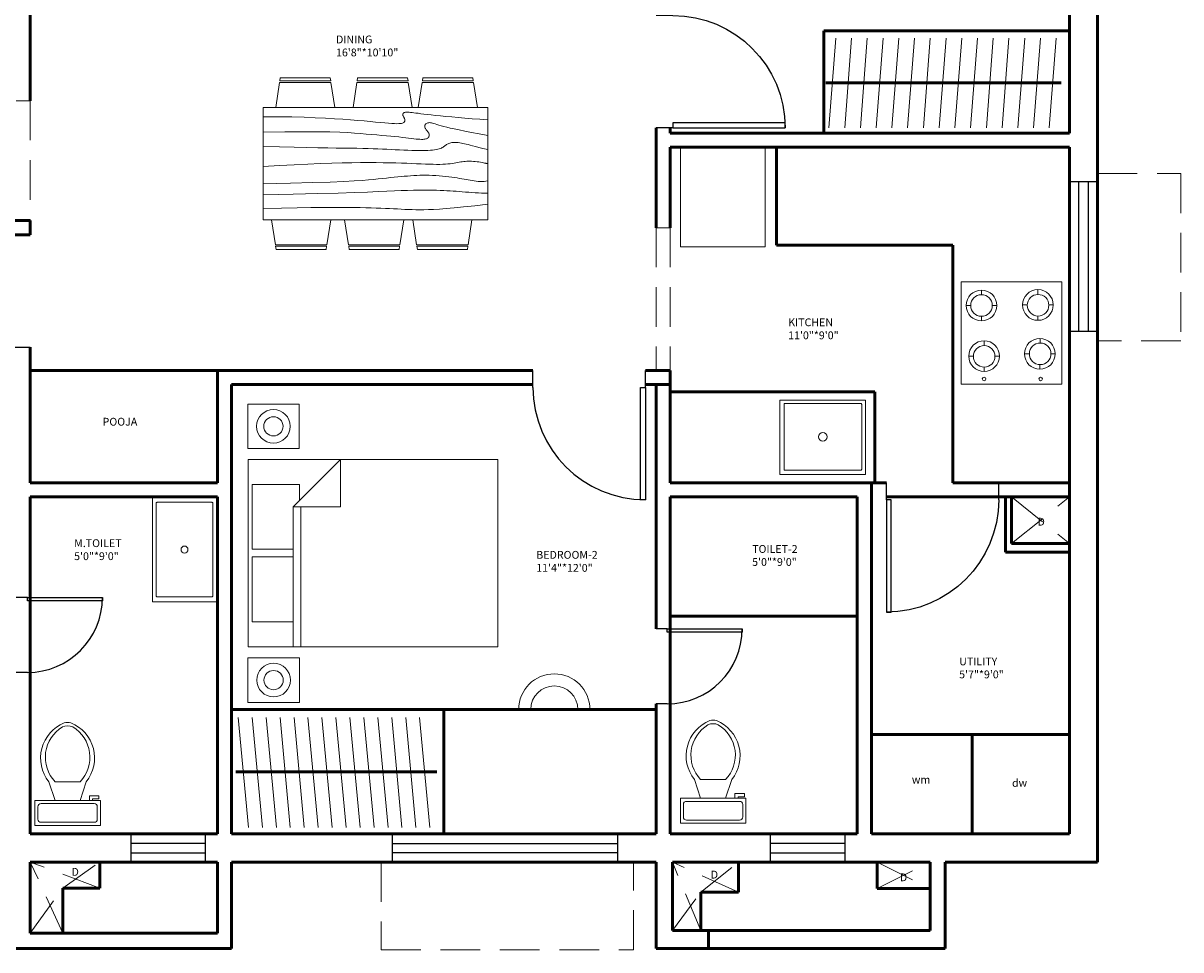
# Model space of a CAD drawing. Units: inches. Extents: x 291 to 2631, y 456 to 2623.
# Tile 21 of 22: x 2205 to 2576, y 2128 to 2425. Entities that reach past the tile are written whole.
import ezdxf

# ---------------------------------------------------------------- set-up
doc = ezdxf.new("R2010")
doc.units = ezdxf.units.IN
doc.linetypes.add('DASHED', pattern=[19.05, 12.7, -6.35])
for name, color, linetype, lineweight in [('A-ANNO-TEXT', 3, 'Continuous', 25), ('A-AREA-IDEN', 7, 'Continuous', 25), ('A-DOOR', 3, 'Continuous', 25), ('A-EQPM', 8, 'Continuous', 18), ('A-FLOR-FIXT', 9, 'Continuous', 18), ('A-FLOR-OVHD', 1, 'DASHED', 18), ('A-FURN', 8, 'Continuous', 18), ('A-GLAZ', 4, 'Continuous', 25), ('A-WALL', 7, 'Continuous', 50)]:
    doc.layers.add(name, color=color, linetype=linetype, lineweight=lineweight)
doc.styles.get("Standard").update_dxf_attribs({"font": 'arial.ttf'})

# ---------------------------------------------------------------- blocks, each defined once
blk = doc.blocks.new('*U2')
for p, q in [((0, 0), (0, -6)), ((40, 0), (40, -6))]:
    blk.add_line(p, q)
blk.add_lwpolyline([(0, 0), (0, 40), (1.75, 40), (1.75, 0)], close=True)
blk.add_arc((0, 0), 40, 0, 90)
blk = doc.blocks.new('Bed - Queen')
for p, q in [((0, -80.00003), (0, 0)), ((0, 0), (59.99999, 0)), ((59.99999, 0), (59.99999, -80.00003)), ((7.99999, -1.2), (28.79998, -1.2)), ((7.99999, -14.4), (7.99999, -1.2)), ((28.79998, -1.2), (28.79998, -14.4)), ((31.19999, -1.2), (51.99999, -1.2)), ((31.19999, -14.4), (31.19999, -1.2)), ((51.99999, -1.2), (51.99999, -16.4)), ((0, -14.4), (44.8, -14.4)), ((59.99999, -29.6), (44.8, -14.4)), ((44.8, -14.4), (44.8, -29.6)), ((44.8, -16.8), (0, -16.8)), ((51.99999, -16.4), (46.79936, -16.4)), ((44.8, -29.6), (59.99999, -29.6)), ((59.99999, -80.00003), (0, -80.00003))]:
    blk.add_line(p, q)
blk = doc.blocks.new('Toilet - top')
for p, q in [((9.5, -6), (9.5, -2)), ((-10, -8.5), (-8, -8.5)), ((-10, -9.5), (-10, -8.5)), ((-7, -9.5), (-10, -9.5)), ((-8, -8.5), (-8, -8)), ((-7, -8), (-7, -9.5)), ((-4, -8), (-6, -14)), ((4, -8), (6, -14)), ((4, -14), (-4, -14))]:
    blk.add_line(p, q)
blk.add_lwpolyline([(10.5, -8), (10.5, 0), (-10.5, 0), (-10.5, -8)], close=True)
for points in [[(-9.5, -2), (-9.5, -6)], [(8.5, -1), (-8.5, -1)], [(-8.5, -7), (8.5, -7)]]:
    blk.add_lwpolyline(points)
for centre, radius, start, end in [((-8.62, -1.88), 0.884, 81.8699, 188.1301), ((8.62, -1.88), 0.884, 351.8699, 98.1301), ((-8.62, -6.12), 0.884, 171.8699, 278.1301), ((8.62, -6.12), 0.884, 261.8699, 8.1301), ((3.52, -21.58), 12.17, 141.4691, 247.9714), ((4.2, -21.82), 11.33, 136.3677, 238.9468), ((-3.52, -21.58), 12.17, 292.0284, 38.5307), ((-4.2, -21.82), 11.33, 301.053, 43.6321), ((0, -27.88), 4, 245.7318, 294.2682), ((0, -29), 4, 254.8605, 285.1395)]:
    blk.add_arc(centre, radius, start, end)
blk = doc.blocks.new('WIN-1800')
for p, q in [((0, 9), (72, 9)), ((0, 0), (0, 9)), ((72, 9), (72, 0)), ((0, 6), (72, 6)), ((72, 3), (0, 3)), ((72, 0), (0, 0))]:
    blk.add_line(p, q)
blk = doc.blocks.new('WIN-1200')
for p, q in [((0, 0), (0, 48)), ((0, 48), (9, 48)), ((3, 0), (3, 48)), ((6, 48), (6, 0)), ((9, 48), (9, 0)), ((9, 0), (0, 0))]:
    blk.add_line(p, q)
blk = doc.blocks.new('COOKTOP')
for p, q in [((6.54, 28.68), (6.54, 30.14)), ((24.62, 30.31), (24.62, 28.76)), ((1.62, 25.22), (3.08, 25.22)), ((10, 25.22), (11.46, 25.22)), ((19.7, 25.39), (21.21, 25.39)), ((28.13, 25.39), (29.54, 25.39)), ((6.54, 21.76), (6.54, 20.3)), ((24.62, 21.83), (24.62, 20.47)), ((7.38, 13.92), (7.38, 12.38)), ((25.35, 14.65), (25.34, 13.21)), ((2.46, 9), (3.95, 9)), ((10.87, 9), (12.3, 9)), ((20.32, 9.73), (21.89, 9.73)), ((28.81, 9.73), (30.16, 9.73)), ((7.38, 5.46), (7.38, 4.08)), ((25.26, 6.28), (25.24, 4.81))]:
    blk.add_line(p, q)
blk.add_lwpolyline([(0, 32.79), (32.25, 32.79), (32.25, 0), (0, 0)], close=True)
for centre, radius in [((6.54, 25.22), 4.92), ((24.62, 25.39), 4.92), ((6.54, 25.22), 3.46), ((24.67, 25.29), 3.46), ((7.38, 9), 4.92), ((7.41, 8.92), 3.46), ((25.24, 9.73), 4.92), ((25.35, 9.74), 3.46), ((7.38, 1.69), 0.572), ((25.5, 1.69), 0.572)]:
    blk.add_circle(centre, radius)
blk = doc.blocks.new('WIN-600')
for p, q in [((24, 9), (0, 9)), ((0, 9), (0, 0)), ((24, 0), (24, 9)), ((24, 6), (0, 6)), ((0, 3), (24, 3)), ((0, 0), (24, 0))]:
    blk.add_line(p, q)

msp = doc.modelspace()

# ---------------------------------------------------------------- linework, layer by layer
at = {"layer": 'A-FLOR-OVHD'}
for p, q in [((2202.49, 2400.18), (2206.99, 2400.18)), ((2206.99, 2400.18), (2206.99, 2361.74)), ((2548.99, 2376.89), (2575.66, 2376.89)), ((2575.66, 2376.89), (2575.66, 2323.27)), ((2407.49, 2359.49), (2411.99, 2359.49)), ((2407.49, 2359.49), (2407.49, 2313.74)), ((2411.99, 2359.49), (2411.99, 2313.74)), ((2575.66, 2323.27), (2548.99, 2323.27)), ((2521.43, 2273.24), (2539.99, 2258.27)), ((2521.43, 2258.27), (2539.99, 2273.24)), ((2217.38, 2133.51), (2206.99, 2156.24)), ((2229.27, 2147.9), (2206.99, 2156.24)), ((2217.38, 2147.9), (2229.27, 2156.24)), ((2319.38, 2156.24), (2319.38, 2128.12)), ((2400.25, 2128.12), (2400.25, 2156.24)), ((2421.83, 2134.3), (2412.72, 2156.24)), ((2433.87, 2146.62), (2412.72, 2156.24)), ((2421.83, 2146.62), (2433.87, 2156.24)), ((2478.37, 2156.24), (2495.34, 2147.73)), ((2478.37, 2147.73), (2495.34, 2156.24)), ((2206.99, 2133.51), (2217.38, 2147.9)), ((2412.72, 2134.3), (2421.83, 2146.62)), ((2319.38, 2128.12), (2400.25, 2128.12))]:
    msp.add_line(p, q, dxfattribs=at)
at = {"layer": 'A-FURN'}
for p, q in [((2462.9, 2391.52), (2465.11, 2420.17)), ((2467.95, 2391.52), (2470.15, 2420.17)), ((2472.99, 2391.52), (2475.2, 2420.17)), ((2478.03, 2391.52), (2480.24, 2420.17)), ((2483.08, 2391.52), (2485.28, 2420.17)), ((2488.12, 2391.52), (2490.33, 2420.17)), ((2493.16, 2391.52), (2495.37, 2420.17)), ((2498.21, 2391.52), (2500.41, 2420.17)), ((2503.25, 2391.52), (2505.46, 2420.17)), ((2508.29, 2391.52), (2510.5, 2420.17)), ((2513.34, 2391.52), (2515.54, 2420.17)), ((2518.38, 2391.52), (2520.59, 2420.17)), ((2523.42, 2391.52), (2525.63, 2420.17)), ((2528.47, 2391.52), (2530.67, 2420.17)), ((2533.51, 2391.52), (2535.72, 2420.17)), ((2287.1, 2407.55), (2286.95, 2406.55)), ((2287.1, 2407.55), (2303.1, 2407.55)), ((2303.26, 2406.55), (2303.1, 2407.55)), ((2311.88, 2407.55), (2311.73, 2406.55)), ((2311.88, 2407.55), (2327.88, 2407.55)), ((2328.04, 2406.55), (2327.88, 2407.55)), ((2332.79, 2407.55), (2332.63, 2406.55)), ((2332.79, 2407.55), (2348.79, 2407.55)), ((2348.94, 2406.55), (2348.79, 2407.55)), ((2286.87, 2406.05), (2285.62, 2398.05)), ((2286.87, 2406.05), (2303.34, 2406.05)), ((2303.26, 2406.55), (2286.95, 2406.55)), ((2304.59, 2398.05), (2303.34, 2406.05)), ((2311.65, 2406.05), (2310.4, 2398.05)), ((2311.65, 2406.05), (2328.12, 2406.05)), ((2328.04, 2406.55), (2311.73, 2406.55)), ((2329.37, 2398.05), (2328.12, 2406.05)), ((2332.55, 2406.05), (2331.3, 2398.05)), ((2332.56, 2406.05), (2349.03, 2406.05)), ((2348.94, 2406.55), (2332.63, 2406.55)), ((2350.27, 2398.05), (2349.02, 2406.05)), ((2353.58, 2398.05), (2281.58, 2398.05)), ((2281.58, 2398.05), (2281.58, 2362.05)), ((2353.58, 2362.05), (2353.58, 2398.05)), ((2281.58, 2362.05), (2353.58, 2362.05)), ((2285.53, 2354.05), (2284.28, 2362.05)), ((2303.25, 2362.05), (2302, 2354.05)), ((2308.94, 2354.05), (2307.69, 2362.05)), ((2326.66, 2362.05), (2325.41, 2354.05)), ((2330.79, 2354.05), (2329.54, 2362.05)), ((2348.51, 2362.05), (2347.26, 2354.05)), ((2285.54, 2354.05), (2302, 2354.05)), ((2285.77, 2352.55), (2285.61, 2353.55)), ((2301.92, 2353.55), (2285.61, 2353.55)), ((2285.77, 2352.55), (2301.77, 2352.55)), ((2301.92, 2353.55), (2301.77, 2352.55)), ((2308.95, 2354.05), (2325.42, 2354.05)), ((2309.18, 2352.55), (2309.02, 2353.55)), ((2325.34, 2353.55), (2309.03, 2353.55)), ((2309.18, 2352.55), (2325.18, 2352.55)), ((2325.34, 2353.55), (2325.18, 2352.55)), ((2330.79, 2354.05), (2347.26, 2354.05)), ((2331.03, 2352.55), (2330.87, 2353.55)), ((2347.18, 2353.55), (2330.87, 2353.55)), ((2331.03, 2352.55), (2347.03, 2352.55)), ((2347.18, 2353.55), (2347.03, 2352.55)), ((2273.61, 2202.53), (2276.89, 2167.35)), ((2278.09, 2202.53), (2281.36, 2167.35)), ((2282.56, 2202.53), (2285.83, 2167.35)), ((2287.03, 2202.53), (2290.3, 2167.35)), ((2291.5, 2202.53), (2294.78, 2167.35)), ((2295.97, 2202.53), (2299.25, 2167.35)), ((2300.44, 2202.53), (2303.72, 2167.35)), ((2304.92, 2202.53), (2308.19, 2167.35)), ((2309.39, 2202.53), (2312.66, 2167.35)), ((2313.86, 2202.53), (2317.13, 2167.35)), ((2318.33, 2202.53), (2321.61, 2167.35)), ((2322.8, 2202.53), (2326.08, 2167.35)), ((2327.28, 2202.53), (2330.55, 2167.35)), ((2331.75, 2202.53), (2335.02, 2167.35))]:
    msp.add_line(p, q, dxfattribs=at)
for points in [[(2281.58, 2395.05), (2286.4, 2395.02), (2290.77, 2394.96), (2294.73, 2394.86), (2298.3, 2394.73), (2301.54, 2394.58), (2304.48, 2394.41), (2307.16, 2394.23), (2309.62, 2394.05), (2311.89, 2393.86), (2313.98, 2393.68), (2315.88, 2393.5), (2317.62, 2393.34), (2319.17, 2393.19), (2320.56, 2393.06), (2321.78, 2392.96), (2322.83, 2392.88), (2323.72, 2392.83), (2324.46, 2392.81), (2325.07, 2392.82), (2325.56, 2392.86), (2325.95, 2392.92), (2326.25, 2393), (2326.48, 2393.1), (2326.66, 2393.21), (2326.8, 2393.34), (2326.9, 2393.49), (2326.97, 2393.64), (2327.01, 2393.81), (2327.02, 2393.97), (2327, 2394.14), (2326.97, 2394.3), (2326.91, 2394.46), (2326.84, 2394.62), (2326.76, 2394.76), (2326.68, 2394.9), (2326.59, 2395.04), (2326.51, 2395.17), (2326.43, 2395.29), (2326.37, 2395.42), (2326.33, 2395.55), (2326.31, 2395.67), (2326.31, 2395.79), (2326.34, 2395.91), (2326.39, 2396.02), (2326.47, 2396.13), (2326.56, 2396.23), (2326.68, 2396.31), (2326.83, 2396.38), (2327, 2396.43), (2327.2, 2396.47), (2327.43, 2396.5), (2327.7, 2396.5), (2328.03, 2396.5), (2328.4, 2396.47), (2328.83, 2396.43), (2329.33, 2396.38), (2329.9, 2396.31), (2330.55, 2396.22), (2331.29, 2396.13), (2332.15, 2396.01), (2333.12, 2395.89), (2334.22, 2395.76), (2335.47, 2395.61), (2336.87, 2395.46), (2338.44, 2395.3), (2340.17, 2395.14), (2342.05, 2394.96), (2344.08, 2394.79), (2346.26, 2394.6), (2348.57, 2394.42), (2351.01, 2394.23), (2353.58, 2394.05)], [(2281.58, 2390.05), (2288.6, 2390.19), (2294.41, 2390.25), (2299.16, 2390.24), (2303.01, 2390.18), (2306.14, 2390.08), (2308.7, 2389.94), (2310.86, 2389.79), (2312.79, 2389.63), (2314.61, 2389.48), (2316.35, 2389.33), (2318.02, 2389.19), (2319.61, 2389.06), (2321.11, 2388.93), (2322.52, 2388.8), (2323.85, 2388.67), (2325.08, 2388.55), (2326.22, 2388.42), (2327.27, 2388.3), (2328.23, 2388.18), (2329.11, 2388.08), (2329.91, 2387.98), (2330.62, 2387.9), (2331.26, 2387.84), (2331.83, 2387.8), (2332.33, 2387.78), (2332.76, 2387.78), (2333.13, 2387.8), (2333.45, 2387.85), (2333.73, 2387.91), (2333.96, 2388), (2334.16, 2388.1), (2334.33, 2388.21), (2334.47, 2388.34), (2334.59, 2388.49), (2334.69, 2388.65), (2334.76, 2388.82), (2334.8, 2388.99), (2334.81, 2389.17), (2334.79, 2389.36), (2334.75, 2389.55), (2334.67, 2389.73), (2334.57, 2389.92), (2334.44, 2390.11), (2334.31, 2390.3), (2334.17, 2390.48), (2334.02, 2390.67), (2333.88, 2390.86), (2333.75, 2391.05), (2333.63, 2391.23), (2333.53, 2391.42), (2333.45, 2391.6), (2333.4, 2391.79), (2333.38, 2391.96), (2333.38, 2392.14), (2333.42, 2392.3), (2333.5, 2392.46), (2333.61, 2392.61), (2333.76, 2392.75), (2333.94, 2392.88), (2334.15, 2392.98), (2334.39, 2393.06), (2334.66, 2393.12), (2334.94, 2393.14), (2335.25, 2393.13), (2335.57, 2393.08), (2335.92, 2392.99), (2336.32, 2392.88), (2336.77, 2392.73), (2337.3, 2392.56), (2337.91, 2392.36), (2338.63, 2392.15), (2339.45, 2391.92), (2340.42, 2391.68), (2341.54, 2391.42), (2342.86, 2391.13), (2344.41, 2390.81), (2346.22, 2390.45), (2348.33, 2390.04), (2350.77, 2389.57), (2353.58, 2389.05)], [(2281.58, 2385.55), (2286.86, 2385.38), (2291.51, 2385.26), (2295.58, 2385.16), (2299.15, 2385.1), (2302.28, 2385.05), (2305.03, 2385.02), (2307.47, 2384.99), (2309.66, 2384.96), (2311.67, 2384.93), (2313.52, 2384.89), (2315.24, 2384.84), (2316.84, 2384.79), (2318.35, 2384.73), (2319.8, 2384.67), (2321.2, 2384.61), (2322.58, 2384.55), (2323.95, 2384.48), (2325.31, 2384.42), (2326.65, 2384.37), (2327.95, 2384.32), (2329.21, 2384.27), (2330.41, 2384.24), (2331.53, 2384.22), (2332.58, 2384.21), (2333.53, 2384.22), (2334.4, 2384.24), (2335.18, 2384.28), (2335.88, 2384.34), (2336.51, 2384.41), (2337.07, 2384.49), (2337.56, 2384.6), (2338, 2384.71), (2338.38, 2384.84), (2338.71, 2384.99), (2339, 2385.14), (2339.27, 2385.31), (2339.51, 2385.47), (2339.73, 2385.64), (2339.95, 2385.8), (2340.16, 2385.96), (2340.39, 2386.11), (2340.62, 2386.26), (2340.87, 2386.39), (2341.13, 2386.5), (2341.42, 2386.61), (2341.72, 2386.69), (2342.05, 2386.75), (2342.41, 2386.8), (2342.8, 2386.82), (2343.22, 2386.81), (2343.67, 2386.79), (2344.13, 2386.74), (2344.62, 2386.68), (2345.12, 2386.6), (2345.64, 2386.5), (2346.16, 2386.38), (2346.7, 2386.25), (2347.29, 2386.09), (2347.95, 2385.92), (2348.71, 2385.71), (2349.63, 2385.48), (2350.72, 2385.21), (2352.03, 2384.9), (2353.58, 2384.55)], [(2281.58, 2379.05), (2286.79, 2379.39), (2291.56, 2379.66), (2295.93, 2379.88), (2299.92, 2380.05), (2303.58, 2380.17), (2306.93, 2380.26), (2310, 2380.31), (2312.83, 2380.34), (2315.45, 2380.34), (2317.87, 2380.33), (2320.11, 2380.31), (2322.19, 2380.27), (2324.13, 2380.22), (2325.94, 2380.17), (2327.64, 2380.11), (2329.25, 2380.05), (2330.77, 2379.98), (2332.21, 2379.92), (2333.58, 2379.87), (2334.86, 2379.83), (2336.06, 2379.79), (2337.18, 2379.78), (2338.21, 2379.78), (2339.16, 2379.8), (2340.03, 2379.84), (2340.82, 2379.9), (2341.53, 2379.98), (2342.19, 2380.07), (2342.8, 2380.16), (2343.37, 2380.26), (2343.9, 2380.37), (2344.41, 2380.46), (2344.91, 2380.55), (2345.39, 2380.63), (2345.87, 2380.7), (2346.35, 2380.75), (2346.84, 2380.79), (2347.34, 2380.81), (2347.86, 2380.82), (2348.41, 2380.8), (2348.99, 2380.75), (2349.58, 2380.69), (2350.17, 2380.62), (2350.74, 2380.54), (2351.28, 2380.45), (2351.77, 2380.36), (2352.19, 2380.28), (2352.54, 2380.21), (2352.79, 2380.16), (2352.96, 2380.12), (2353.08, 2380.09), (2353.17, 2380.07), (2353.24, 2380.05), (2353.32, 2380.05), (2353.42, 2380.05), (2353.58, 2380.05)], [(2281.58, 2373.55), (2290.4, 2373.73), (2297.5, 2373.92), (2303.11, 2374.1), (2307.47, 2374.29), (2310.8, 2374.46), (2313.34, 2374.64), (2315.32, 2374.8), (2316.95, 2374.96), (2318.45, 2375.11), (2319.85, 2375.26), (2321.17, 2375.4), (2322.41, 2375.52), (2323.58, 2375.65), (2324.71, 2375.76), (2325.78, 2375.86), (2326.83, 2375.96), (2327.85, 2376.05), (2328.85, 2376.13), (2329.84, 2376.2), (2330.83, 2376.25), (2331.81, 2376.29), (2332.81, 2376.31), (2333.81, 2376.32), (2334.83, 2376.3), (2335.87, 2376.25), (2336.92, 2376.19), (2337.98, 2376.11), (2339.03, 2376.01), (2340.05, 2375.91), (2341.05, 2375.79), (2342.01, 2375.67), (2342.91, 2375.55), (2343.76, 2375.42), (2344.55, 2375.3), (2345.29, 2375.17), (2346, 2375.05), (2346.68, 2374.93), (2347.34, 2374.81), (2347.98, 2374.7), (2348.62, 2374.59), (2349.26, 2374.48), (2349.91, 2374.39), (2350.55, 2374.31), (2351.18, 2374.27), (2351.8, 2374.26), (2352.41, 2374.3), (2353.01, 2374.39), (2353.58, 2374.55)], [(2281.58, 2370.05), (2291.18, 2370.23), (2299.11, 2370.42), (2305.6, 2370.6), (2310.84, 2370.76), (2315.06, 2370.92), (2318.46, 2371.07), (2321.26, 2371.19), (2323.66, 2371.3), (2325.86, 2371.38), (2327.88, 2371.44), (2329.75, 2371.48), (2331.48, 2371.5), (2333.07, 2371.51), (2334.54, 2371.51), (2335.9, 2371.49), (2337.16, 2371.46), (2338.34, 2371.43), (2339.45, 2371.39), (2340.5, 2371.34), (2341.51, 2371.28), (2342.49, 2371.22), (2343.46, 2371.15), (2344.43, 2371.08), (2345.41, 2371), (2346.43, 2370.92), (2347.46, 2370.84), (2348.51, 2370.77), (2349.56, 2370.7), (2350.6, 2370.64), (2351.62, 2370.59), (2352.62, 2370.56), (2353.58, 2370.55)], [(2281.58, 2365.55), (2287.49, 2365.71), (2292.55, 2365.83), (2296.85, 2365.92), (2300.5, 2365.97), (2303.61, 2366), (2306.28, 2366), (2308.61, 2365.99), (2310.7, 2365.96), (2312.66, 2365.93), (2314.49, 2365.89), (2316.21, 2365.84), (2317.82, 2365.79), (2319.34, 2365.73), (2320.78, 2365.67), (2322.13, 2365.61), (2323.41, 2365.55), (2324.63, 2365.48), (2325.81, 2365.42), (2326.97, 2365.37), (2328.13, 2365.32), (2329.3, 2365.28), (2330.51, 2365.26), (2331.78, 2365.25), (2333.12, 2365.25), (2334.57, 2365.28), (2336.19, 2365.34), (2338.06, 2365.44), (2340.24, 2365.6), (2342.81, 2365.83), (2345.84, 2366.14), (2349.41, 2366.54), (2353.58, 2367.05)]]:
    msp.add_lwpolyline(points, dxfattribs=at)
for points in [[(2415.32, 2385.24), (2442.51, 2385.24), (2442.51, 2353.36), (2415.32, 2353.36)], [(2447.16, 2304.27), (2474.6, 2304.27), (2474.6, 2280.37), (2447.16, 2280.37)], [(2276.65, 2303), (2293.13, 2303), (2293.13, 2288.7), (2276.65, 2288.7)], [(2266.99, 2273.24), (2246.11, 2273.24), (2246.11, 2239.58), (2266.99, 2239.58)], [(2276.71, 2221.69), (2293.2, 2221.69), (2293.2, 2207.39), (2276.71, 2207.39)]]:
    msp.add_lwpolyline(points, close=True, dxfattribs=at)
for points in [[(2448.8, 2303.16), (2473.1, 2303.16, -0.414214), (2473.4, 2302.86), (2473.4, 2282.08, -0.414214), (2473.1, 2281.78), (2448.8, 2281.78, -0.414214), (2448.5, 2282.08), (2448.5, 2302.86, -0.414214)], [(2247.64, 2271.51), (2265.17, 2271.51, -0.414214), (2265.47, 2271.21), (2265.47, 2241.53, -0.414214), (2265.17, 2241.23), (2247.64, 2241.23, -0.414214), (2247.34, 2241.53), (2247.34, 2271.21, -0.414214)]]:
    msp.add_lwpolyline(points, format="xyb", close=True, dxfattribs=at)
for centre, radius in [((2284.89, 2295.85), 5.39), ((2284.89, 2295.85), 3.08), ((2460.95, 2292.47), 1.36), ((2256.4, 2256.37), 1.12), ((2284.95, 2214.54), 5.39), ((2284.95, 2214.54), 3.08)]:
    msp.add_circle(centre, radius, dxfattribs=at)
for radius in [11.41, 7.54]:
    msp.add_arc((2374.9, 2205.13), radius, 0, 180, dxfattribs=at)
at = {"layer": 'A-WALL'}
for p, q in [((2548.99, 2558.74), (2548.99, 2156.24)), ((2539.99, 2549.74), (2539.99, 2389.74)), ((2206.99, 2525.27), (2206.99, 2400.18)), ((2461.25, 2389.74), (2461.25, 2422.59)), ((2461.25, 2422.59), (2539.99, 2422.59)), ((2461.92, 2405.85), (2537.36, 2405.85)), ((2407.49, 2359.49), (2407.49, 2391.48)), ((2411.99, 2389.74), (2411.99, 2391.48)), ((2411.99, 2389.74), (2539.99, 2389.74)), ((2411.99, 2359.49), (2411.99, 2385.24)), ((2411.99, 2385.24), (2539.99, 2385.24)), ((2446.06, 2385.24), (2446.06, 2353.91)), ((2539.99, 2385.24), (2539.99, 2165.24)), ((2068.49, 2361.74), (2206.99, 2361.74)), ((2206.99, 2361.74), (2206.99, 2357.24)), ((2068.49, 2357.24), (2206.99, 2357.24)), ((2446.06, 2353.91), (2502.57, 2353.91)), ((2502.57, 2353.91), (2502.57, 2277.74)), ((2206.99, 2321.24), (2206.99, 2277.74)), ((2206.99, 2313.74), (2368.07, 2313.74)), ((2266.99, 2313.74), (2266.99, 2277.74)), ((2404.07, 2313.74), (2411.99, 2313.74)), ((2411.99, 2313.74), (2411.99, 2277.74)), ((2271.49, 2309.24), (2271.49, 2165.24)), ((2271.49, 2309.24), (2368.07, 2309.24)), ((2404.07, 2309.24), (2411.99, 2309.24)), ((2407.49, 2309.24), (2407.49, 2230.94)), ((2411.99, 2306.92), (2477.59, 2306.92)), ((2477.59, 2306.92), (2477.59, 2277.74)), ((2206.99, 2277.74), (2266.99, 2277.74)), ((2411.99, 2277.74), (2481.3, 2277.74)), ((2476.49, 2277.74), (2476.49, 2165.24)), ((2502.57, 2277.74), (2539.99, 2277.74)), ((2206.99, 2273.24), (2266.99, 2273.24)), ((2206.99, 2273.24), (2206.99, 2165.24)), ((2266.99, 2273.24), (2266.99, 2165.24)), ((2411.99, 2273.24), (2471.99, 2273.24)), ((2411.99, 2273.24), (2411.99, 2165.24)), ((2471.99, 2273.24), (2471.99, 2165.24)), ((2481.3, 2273.24), (2539.99, 2273.24)), ((2519.46, 2273.24), (2519.46, 2255.51)), ((2521.43, 2273.24), (2521.43, 2258.27)), ((2519.46, 2255.51), (2539.99, 2255.51)), ((2521.43, 2258.27), (2539.99, 2258.27)), ((2411.99, 2234.99), (2471.99, 2234.99)), ((2271.49, 2205.13), (2407.49, 2205.13)), ((2339.49, 2205.13), (2339.49, 2165.24)), ((2407.49, 2206.94), (2407.49, 2165.24)), ((2476.49, 2197.06), (2539.99, 2197.06)), ((2508.84, 2197.06), (2508.84, 2165.24)), ((2272.85, 2185.1), (2337.28, 2185.1)), ((2206.99, 2165.24), (2266.99, 2165.24)), ((2271.49, 2165.24), (2407.49, 2165.24)), ((2411.99, 2165.24), (2471.99, 2165.24)), ((2476.49, 2165.24), (2539.99, 2165.24)), ((2206.99, 2156.24), (2206.99, 2133.51)), ((2206.99, 2156.24), (2266.99, 2156.24)), ((2229.27, 2147.9), (2229.27, 2156.24)), ((2266.99, 2133.51), (2266.99, 2156.24)), ((2271.49, 2128.54), (2271.49, 2156.24)), ((2271.49, 2156.24), (2407.49, 2156.24)), ((2407.49, 2156.24), (2407.49, 2128.54)), ((2412.72, 2156.24), (2412.72, 2134.3)), ((2412.72, 2156.24), (2495.34, 2156.24)), ((2433.87, 2146.62), (2433.87, 2156.24)), ((2478.37, 2156.24), (2478.37, 2147.73)), ((2495.34, 2134.3), (2495.34, 2156.24)), ((2500.12, 2128.54), (2500.12, 2156.24)), ((2500.12, 2156.24), (2548.99, 2156.24)), ((2217.38, 2133.51), (2217.38, 2147.9)), ((2217.38, 2147.9), (2229.27, 2147.9)), ((2421.83, 2134.3), (2421.83, 2146.62)), ((2421.83, 2146.62), (2433.87, 2146.62)), ((2478.37, 2147.73), (2495.34, 2147.73)), ((2206.99, 2133.51), (2266.99, 2133.51)), ((2412.72, 2134.3), (2495.34, 2134.3)), ((2424.31, 2134.3), (2424.31, 2128.54)), ((2202.49, 2128.54), (2271.49, 2128.54)), ((2407.49, 2128.54), (2500.12, 2128.54))]:
    msp.add_line(p, q, dxfattribs=at)

# ---------------------------------------------------------------- block references
at = {"layer": 'A-DOOR'}
for p, xscale, yscale, zscale, rotation in [((2412.89, 2391.48), -0.9, 0.9, 0.9, 270), ((2201.59, 2357.24), -0.9, 0.9, 0.9, 90), ((2404.07, 2308.34), 0.9, 0.9, 0.9, 180), ((2481.3, 2272.34), -0.9, 0.9, 0.9, 180), ((2206.09, 2241), 0.6, 0.6, 0.6, 270), ((2411.09, 2230.94), 0.6, 0.6, 0.6, 270)]:
    msp.add_blockref('*U2', p, dxfattribs=dict(at, xscale=xscale, yscale=yscale, zscale=zscale, rotation=rotation))
at = {"layer": 'A-EQPM'}
msp.add_blockref('COOKTOP', (2505.24, 2309.34), dxfattribs=at)
at = {"layer": 'A-FLOR-FIXT', "rotation": 180}
for p in [(2218.94, 2167.99), (2425.79, 2168.69)]:
    msp.add_blockref('Toilet - top', p, dxfattribs=at)
at = {"layer": 'A-FURN', "rotation": 90}
msp.add_blockref('Bed - Queen', (2276.83, 2225.24), dxfattribs=at)
at = {"layer": 'A-GLAZ'}
for name, p in [('WIN-1200', (2539.99, 2326.28)), ('WIN-600', (2239.18, 2156.24)), ('WIN-1800', (2323.1, 2156.24))]:
    msp.add_blockref(name, p, dxfattribs=at)
at = {"layer": 'A-GLAZ', "rotation": 180}
msp.add_blockref('WIN-600', (2468.08, 2165.24), dxfattribs=at)

# ---------------------------------------------------------------- texts
at = {"layer": 'A-ANNO-TEXT', "char_height": 2.5, "attachment_point": 1}
for s, width, insert in [('D', 2.7166, (2529.74, 2266.53)), ('wm', 24.9352, (2489.47, 2183.89)), ('dw', 14.5822, (2521.56, 2182.86)), ('D', 3.1099, (2220.21, 2154.35)), ('D', 1.5733, (2425.02, 2153.47)), ('D', 2.1765, (2485.63, 2152.6))]:
    msp.add_mtext_dynamic_manual_height_columns(s, width=width, gutter_width=12.5, heights=[0], dxfattribs=dict(at, insert=insert))
at = {"layer": 'A-AREA-IDEN', "char_height": 2.5, "attachment_point": 1}
for s, width, insert in [('DINING\\P16\'8"*10\'10"', 50.7137, (2304.95, 2421.05)), ('KITCHEN\\P11\'0"*9\'0"', 58.1136, (2449.83, 2330.42)), ('POOJA', 41.6262, (2230.16, 2298.57)), ('M.TOILET\\P5\'0"*9\'0"', 31.7479, (2221.04, 2259.66)), ('BEDROOM-2\\P11\'4"*12\'0"', 40.0049, (2369.12, 2255.92)), ('TOILET-2\\P5\'0"*9\'0"', 43.159, (2438.3, 2257.8)), ('UTILITY\\P5\'7"*9\'0"', 46.6063, (2504.63, 2221.78))]:
    msp.add_mtext_dynamic_manual_height_columns(s, width=width, gutter_width=12.5, heights=[0], dxfattribs=dict(at, insert=insert))

doc.saveas('drawing.dxf')
